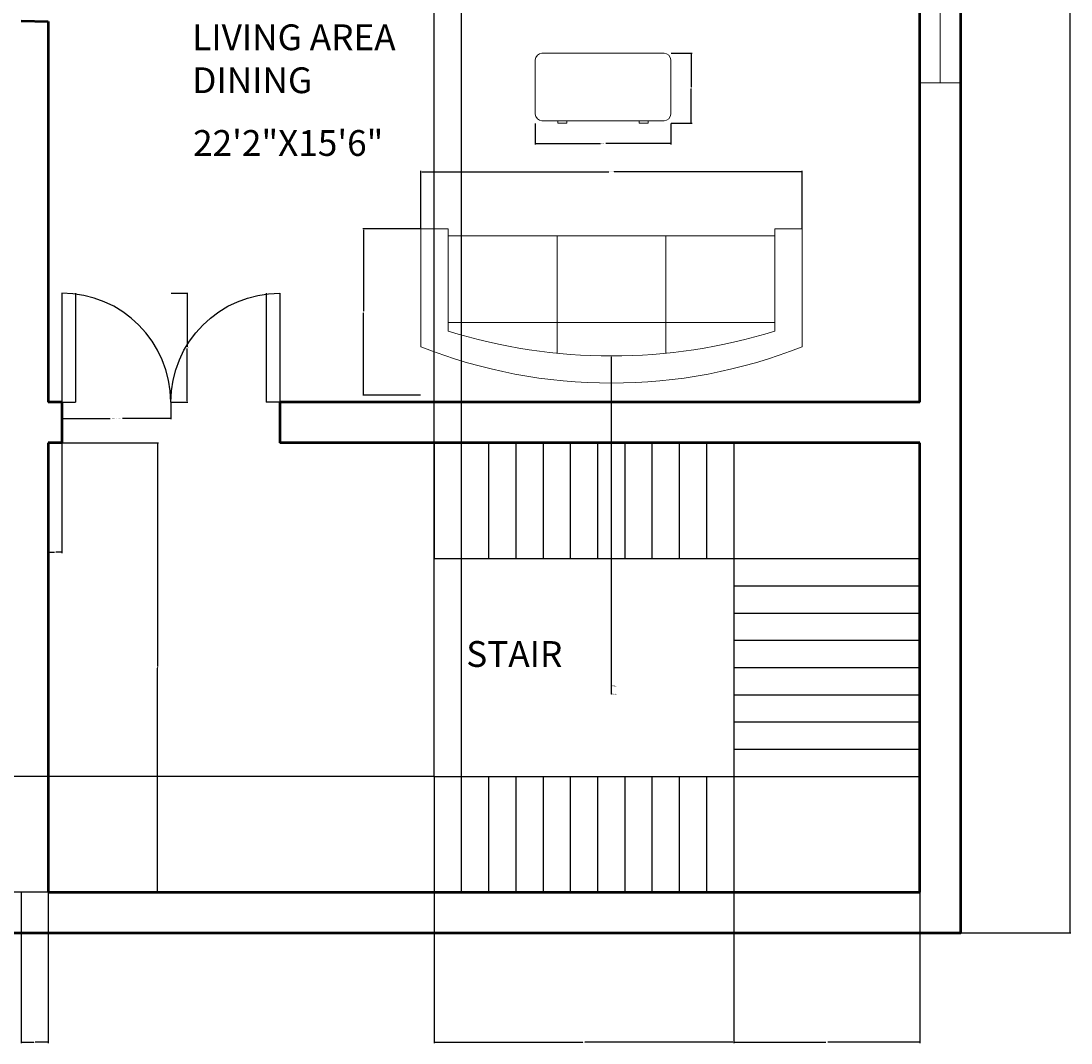
# Model space of a CAD drawing. Units: inches. Extents: x 66 to 499, y 601 to 1111.
# Tile 2 of 4: x 268 to 499, y 601 to 826. Entities that reach past the tile are written whole.
import ezdxf

# ---------------------------------------------------------------- set-up
doc = ezdxf.new("R2010")
doc.units = ezdxf.units.IN
for name, color, linetype, lineweight in [('A-ANNO-DIMS', 2, 'Continuous', 18), ('A-AREA-IDEN', 7, 'Continuous', 18), ('A-DOOR', 3, 'Continuous', 25), ('A-FLOR-STRS', 7, 'Continuous', 25), ('A-FURN', 8, 'Continuous', 18), ('A-GLAZ', 4, 'Continuous', 18), ('A-WALL', 7, 'Continuous', 50)]:
    doc.layers.add(name, color=color, linetype=linetype, lineweight=lineweight)
doc.styles.get("Standard").update_dxf_attribs({"font": 'arial.ttf'})
doc.dimstyles.get("Standard").update_dxf_attribs({"dimtxt": 0.18, "dimasz": 0.18, "dimexe": 0.18, "dimexo": 0.0625, "dimgap": 0.09, "dimtad": 0, "dimtih": 1, "dimtoh": 1, "dimdec": 4, "dimzin": 0, "dimdsep": 46, "dimtxsty": 'Standard', "dimcen": 0.09, "dimadec": 0, "dimazin": 0, "dimtfac": 1, "dimtdec": 4, "dimtofl": 0, "dimtmove": 0, "dimatfit": 3, "dimfxl": 1, "dimtolj": 1, "dimtzin": 0, "dimarcsym": 0})

# ---------------------------------------------------------------- blocks, each defined once
blk = doc.blocks.new('Sofa - Roundback 7 ft.')
for p, q in [((-12.00002, -32.4421), (-12.00003, -6.5971)), ((11.99997, -32.4421), (11.99998, -6.5971)), ((-36.000027, -34), (-36.000027, -11.4696)), ((35.99998, -34), (35.99998, -11.4696)), ((-35.999844, -13.3819), (35.9998, -13.3819)), ((-36.000027, -32.4421), (35.99998, -32.4421))]:
    blk.add_line(p, q)
for points in [[(-36.000027, -34), (-42.000027, -34), (-42.000027, -8)], [(41.99998, -8), (41.99998, -34), (35.99998, -34)]]:
    blk.add_lwpolyline(points)
for centre, radius, start, end in [((0, -114.25), 114.25, 68.43141, 111.5686), ((-0.00001, -127.1968), 121.1968, 72.72033, 107.2797)]:
    blk.add_arc(centre, radius, start, end)
blk = doc.blocks.new('Desk - 30 x 60 in.')
for p, q in [((-26.999995, 0), (26.999995, 0)), ((-29.999995, -27), (-29.999995, -3)), ((29.999995, -3), (29.999995, -27)), ((26.999995, -30), (-26.999995, -30)), ((-20.000005, -30), (-20.000005, -31)), ((-20.000005, -31), (-16.000005, -31)), ((-16.000005, -31), (-16.000005, -30)), ((15.999995, -31), (15.999995, -30)), ((19.999995, -31), (15.999995, -31)), ((19.999995, -30), (19.999995, -31))]:
    blk.add_line(p, q)
for centre, start, end in [((-26.499995, -3.5), 98.1301, 171.8699), ((26.499995, -3.5), 8.130102, 81.8699), ((-26.499995, -26.5), 188.1301, 261.8699), ((26.499995, -26.5), 278.1301, 351.8699)]:
    blk.add_arc(centre, 3.535534, start, end)
blk = doc.blocks.new('DOOR-LEAF-24IN')
for p, q in [((0, 24), (0, 0)), ((3, 24), (3, 0)), ((0, 0), (3, 0))]:
    blk.add_line(p, q)
blk.add_arc((0, 0), 24, 0, 90)
blk = doc.blocks.new('WIN-60IN')
for p, q in [((60, 9), (0, 9)), ((0, 9), (0, 0)), ((60, 0), (60, 9)), ((0, 4.5), (60, 4.5)), ((0, 0), (60, 0))]:
    blk.add_line(p, q)
blk = doc.blocks.new('*D28')
at = {"layer": 'A-ANNO-DIMS', "color": 0, "lineweight": -2, "transparency": 16777216}
for p, q in [((276.58, 741.94), (276.58, 738.22)), ((300.58, 741.94), (300.58, 738.22)), ((276.76, 738.4), (287.24, 738.4)), ((300.4, 738.4), (289.91, 738.4))]:
    blk.add_line(p, q, dxfattribs=at)
at = {"layer": 'A-ANNO-DIMS', "color": 0, "transparency": 16777216}
for points in [[(276.76, 738.43), (276.76, 738.37), (276.58, 738.4)], [(300.4, 738.43), (300.4, 738.37), (300.58, 738.4)]]:
    blk.add_solid(points, dxfattribs=at)
at = {"layer": 'Defpoints', "color": 0, "transparency": 16777216}
for p in [(276.58, 742), (300.58, 742), (300.58, 738.4)]:
    blk.add_point(p, dxfattribs=at)
at = {"layer": 'A-ANNO-DIMS', "color": 0, "transparency": 16777216, "insert": (288.58, 738.4), "char_height": 0.18, "attachment_point": 5}
blk.add_mtext('\\A1;ENTRY LEAF 24 TYP.', dxfattribs=at)
blk = doc.blocks.new('*D29')
at = {"layer": 'A-ANNO-DIMS', "color": 0, "lineweight": -2, "transparency": 16777216}
for p, q in [((300.64, 766), (304.36, 766)), ((304.18, 765.82), (304.18, 754.18)), ((304.18, 742.18), (304.18, 753.82)), ((300.64, 742), (304.36, 742))]:
    blk.add_line(p, q, dxfattribs=at)
at = {"layer": 'A-ANNO-DIMS', "color": 0, "transparency": 16777216}
for points in [[(304.15, 765.82), (304.21, 765.82), (304.18, 766)], [(304.15, 742.18), (304.21, 742.18), (304.18, 742)]]:
    blk.add_solid(points, dxfattribs=at)
at = {"layer": 'Defpoints', "color": 0, "transparency": 16777216}
for p in [(300.58, 766), (304.18, 766), (300.58, 742)]:
    blk.add_point(p, dxfattribs=at)
at = {"layer": 'A-ANNO-DIMS', "color": 0, "transparency": 16777216, "insert": (304.18, 754), "char_height": 0.18, "attachment_point": 5}
blk.add_mtext('\\A1;24 TYP.', dxfattribs=at)
blk = doc.blocks.new('*D34')
at = {"layer": 'A-ANNO-DIMS', "color": 0, "lineweight": -2, "transparency": 16777216}
for p, q in [((355.66, 780.24), (355.66, 792.96)), ((355.84, 792.78), (397.06, 792.78)), ((439.48, 792.78), (398.25, 792.78)), ((439.66, 780.24), (439.66, 792.96))]:
    blk.add_line(p, q, dxfattribs=at)
at = {"layer": 'A-ANNO-DIMS', "color": 0, "transparency": 16777216}
for points in [[(355.84, 792.81), (355.84, 792.75), (355.66, 792.78)], [(439.48, 792.81), (439.48, 792.75), (439.66, 792.78)]]:
    blk.add_solid(points, dxfattribs=at)
at = {"layer": 'Defpoints', "color": 0, "transparency": 16777216}
for p in [(355.66, 792.78), (355.66, 780.18), (439.66, 780.18)]:
    blk.add_point(p, dxfattribs=at)
at = {"layer": 'A-ANNO-DIMS', "color": 0, "transparency": 16777216, "insert": (397.66, 792.78), "char_height": 0.18, "attachment_point": 5}
blk.add_mtext('\\A1;SOFA 84', dxfattribs=at)
blk = doc.blocks.new('*D35')
at = {"layer": 'A-ANNO-DIMS', "color": 0, "lineweight": -2, "transparency": 16777216}
for p, q in [((355.59, 780.18), (342.88, 780.18)), ((343.06, 780), (343.06, 762.03)), ((343.06, 743.7), (343.06, 761.67)), ((355.59, 743.52), (342.88, 743.52))]:
    blk.add_line(p, q, dxfattribs=at)
at = {"layer": 'A-ANNO-DIMS', "color": 0, "transparency": 16777216}
for points in [[(343.03, 780), (343.09, 780), (343.06, 780.18)], [(343.03, 743.7), (343.09, 743.7), (343.06, 743.52)]]:
    blk.add_solid(points, dxfattribs=at)
at = {"layer": 'Defpoints', "color": 0, "transparency": 16777216}
for p in [(355.66, 780.18), (343.06, 743.52), (355.66, 743.52)]:
    blk.add_point(p, dxfattribs=at)
at = {"layer": 'A-ANNO-DIMS', "color": 0, "transparency": 16777216, "insert": (343.06, 761.85), "char_height": 0.18, "attachment_point": 5}
blk.add_mtext('\\A1;37', dxfattribs=at)
blk = doc.blocks.new('*D36')
at = {"layer": 'A-ANNO-DIMS', "color": 0, "lineweight": -2, "transparency": 16777216}
for p, q in [((380.82, 803.4), (380.82, 798.8)), ((410.75, 803.4), (410.75, 798.8)), ((381, 798.98), (395.2, 798.98)), ((410.57, 798.98), (396.38, 798.98))]:
    blk.add_line(p, q, dxfattribs=at)
at = {"layer": 'A-ANNO-DIMS', "color": 0, "transparency": 16777216}
for points in [[(381, 799.01), (381, 798.95), (380.82, 798.98)], [(410.57, 799.01), (410.57, 798.95), (410.75, 798.98)]]:
    blk.add_solid(points, dxfattribs=at)
at = {"layer": 'Defpoints', "color": 0, "transparency": 16777216}
for p in [(380.82, 803.47), (410.75, 803.47), (410.75, 798.98)]:
    blk.add_point(p, dxfattribs=at)
at = {"layer": 'A-ANNO-DIMS', "color": 0, "transparency": 16777216, "insert": (395.79, 798.98), "char_height": 0.18, "attachment_point": 5}
blk.add_mtext('\\A1;DESK 30', dxfattribs=at)
blk = doc.blocks.new('*D37')
at = {"layer": 'A-ANNO-DIMS', "color": 0, "lineweight": -2, "transparency": 16777216}
for p, q in [((410.82, 818.93), (415.42, 818.93)), ((415.24, 818.75), (415.24, 811.38)), ((415.24, 803.65), (415.24, 811.02)), ((410.82, 803.47), (415.42, 803.47))]:
    blk.add_line(p, q, dxfattribs=at)
at = {"layer": 'A-ANNO-DIMS', "color": 0, "transparency": 16777216}
for points in [[(415.21, 818.75), (415.27, 818.75), (415.24, 818.93)], [(415.21, 803.65), (415.27, 803.65), (415.24, 803.47)]]:
    blk.add_solid(points, dxfattribs=at)
at = {"layer": 'Defpoints', "color": 0, "transparency": 16777216}
for p in [(410.75, 818.93), (415.24, 818.93), (410.75, 803.47)]:
    blk.add_point(p, dxfattribs=at)
at = {"layer": 'A-ANNO-DIMS', "color": 0, "transparency": 16777216, "insert": (415.24, 811.2), "char_height": 0.18, "attachment_point": 5}
blk.add_mtext('\\A1;15', dxfattribs=at)
blk = doc.blocks.new('*D43')
at = {"layer": 'A-ANNO-DIMS', "color": 0, "lineweight": -2, "transparency": 16777216}
for p, q in [((474.64, 1087), (498.86, 1087)), ((498.68, 1086.82), (498.68, 856.19)), ((498.68, 625.18), (498.68, 855.82)), ((474.64, 625), (498.86, 625))]:
    blk.add_line(p, q, dxfattribs=at)
at = {"layer": 'A-ANNO-DIMS', "color": 0, "transparency": 16777216}
for points in [[(498.65, 1086.82), (498.71, 1086.82), (498.68, 1087)], [(498.65, 625.18), (498.71, 625.18), (498.68, 625)]]:
    blk.add_solid(points, dxfattribs=at)
at = {"layer": 'Defpoints', "color": 0, "transparency": 16777216}
for p in [(474.58, 1087), (498.68, 1087), (474.58, 625)]:
    blk.add_point(p, dxfattribs=at)
at = {"layer": 'A-ANNO-DIMS', "color": 0, "transparency": 16777216, "insert": (498.68, 856), "char_height": 0.18, "attachment_point": 5}
blk.add_mtext('\\A1;462', dxfattribs=at)
blk = doc.blocks.new('*D51')
at = {"layer": 'A-ANNO-DIMS', "color": 0, "lineweight": -2, "transparency": 16777216}
for p, q in [((273.64, 733), (297.86, 733)), ((297.68, 732.82), (297.68, 683.69)), ((297.68, 634.18), (297.68, 683.32)), ((273.64, 634), (297.86, 634))]:
    blk.add_line(p, q, dxfattribs=at)
at = {"layer": 'A-ANNO-DIMS', "color": 0, "transparency": 16777216}
for points in [[(297.65, 732.82), (297.71, 732.82), (297.68, 733)], [(297.65, 634.18), (297.71, 634.18), (297.68, 634)]]:
    blk.add_solid(points, dxfattribs=at)
at = {"layer": 'Defpoints', "color": 0, "transparency": 16777216}
for p in [(273.58, 733), (273.58, 634), (297.68, 634)]:
    blk.add_point(p, dxfattribs=at)
at = {"layer": 'A-ANNO-DIMS', "color": 0, "transparency": 16777216, "insert": (297.68, 683.5), "char_height": 0.18, "attachment_point": 5}
blk.add_mtext('\\A1;99', dxfattribs=at)
blk = doc.blocks.new('*D52')
at = {"layer": 'A-ANNO-DIMS', "color": 0, "lineweight": -2, "transparency": 16777216}
for p, q in [((358.58, 633.94), (358.58, 600.72)), ((424.58, 633.94), (424.58, 600.72)), ((358.76, 600.9), (391.36, 600.9)), ((424.4, 600.9), (391.8, 600.9))]:
    blk.add_line(p, q, dxfattribs=at)
at = {"layer": 'A-ANNO-DIMS', "color": 0, "transparency": 16777216}
for points in [[(358.76, 600.93), (358.76, 600.87), (358.58, 600.9)], [(424.4, 600.93), (424.4, 600.87), (424.58, 600.9)]]:
    blk.add_solid(points, dxfattribs=at)
at = {"layer": 'Defpoints', "color": 0, "transparency": 16777216}
for p in [(358.58, 634), (424.58, 634), (424.58, 600.9)]:
    blk.add_point(p, dxfattribs=at)
at = {"layer": 'A-ANNO-DIMS', "color": 0, "transparency": 16777216, "insert": (391.58, 600.9), "char_height": 0.18, "attachment_point": 5}
blk.add_mtext('\\A1;66', dxfattribs=at)
blk = doc.blocks.new('*D53')
at = {"layer": 'A-ANNO-DIMS', "color": 0, "lineweight": -2, "transparency": 16777216}
for p, q in [((424.58, 633.94), (424.58, 600.72)), ((465.58, 633.94), (465.58, 600.72)), ((424.76, 600.9), (444.87, 600.9)), ((465.4, 600.9), (445.28, 600.9))]:
    blk.add_line(p, q, dxfattribs=at)
at = {"layer": 'A-ANNO-DIMS', "color": 0, "transparency": 16777216}
for points in [[(424.76, 600.93), (424.76, 600.87), (424.58, 600.9)], [(465.4, 600.93), (465.4, 600.87), (465.58, 600.9)]]:
    blk.add_solid(points, dxfattribs=at)
at = {"layer": 'Defpoints', "color": 0, "transparency": 16777216}
for p in [(424.58, 634), (465.58, 634), (465.58, 600.9)]:
    blk.add_point(p, dxfattribs=at)
at = {"layer": 'A-ANNO-DIMS', "color": 0, "transparency": 16777216, "insert": (445.08, 600.9), "char_height": 0.18, "attachment_point": 5}
blk.add_mtext('\\A1;41', dxfattribs=at)
blk = doc.blocks.new('*D54')
at = {"layer": 'A-ANNO-DIMS', "color": 0, "lineweight": -2, "transparency": 16777216}
for p, q in [((358.51, 659.5), (66.3, 659.5)), ((66.48, 659.32), (66.48, 646.94)), ((66.48, 634.18), (66.48, 646.57)), ((358.51, 634), (66.3, 634))]:
    blk.add_line(p, q, dxfattribs=at)
at = {"layer": 'A-ANNO-DIMS', "color": 0, "transparency": 16777216}
for points in [[(66.45, 659.32), (66.51, 659.32), (66.48, 659.5)], [(66.45, 634.18), (66.51, 634.18), (66.48, 634)]]:
    blk.add_solid(points, dxfattribs=at)
at = {"layer": 'Defpoints', "color": 0, "transparency": 16777216}
for p in [(66.48, 659.5), (358.58, 659.5), (358.58, 634)]:
    blk.add_point(p, dxfattribs=at)
at = {"layer": 'A-ANNO-DIMS', "color": 0, "transparency": 16777216, "insert": (66.48, 646.75), "char_height": 0.18, "attachment_point": 5}
blk.add_mtext('\\A1;25.5', dxfattribs=at)
blk = doc.blocks.new('*D55')
at = {"layer": 'A-ANNO-DIMS', "color": 0, "lineweight": -2, "transparency": 16777216}
for p, q in [((358.58, 659.57), (358.58, 1111.28)), ((358.76, 1111.1), (361.43, 1111.1)), ((364.4, 1111.1), (361.73, 1111.1)), ((364.58, 659.57), (364.58, 1111.28))]:
    blk.add_line(p, q, dxfattribs=at)
at = {"layer": 'A-ANNO-DIMS', "color": 0, "transparency": 16777216}
for points in [[(358.76, 1111.13), (358.76, 1111.07), (358.58, 1111.1)], [(364.4, 1111.13), (364.4, 1111.07), (364.58, 1111.1)]]:
    blk.add_solid(points, dxfattribs=at)
at = {"layer": 'Defpoints', "color": 0, "transparency": 16777216}
for p in [(364.58, 1111.1), (358.58, 659.5), (364.58, 659.5)]:
    blk.add_point(p, dxfattribs=at)
at = {"layer": 'A-ANNO-DIMS', "color": 0, "transparency": 16777216, "insert": (361.58, 1111.1), "char_height": 0.18, "attachment_point": 5}
blk.add_mtext('\\A1;6', dxfattribs=at)
blk = doc.blocks.new('*D62')
at = {"layer": 'A-ANNO-DIMS', "color": 0, "lineweight": -2, "transparency": 16777216}
for p, q in [((267.58, 633.94), (267.58, 600.72)), ((273.58, 633.94), (273.58, 600.72)), ((267.76, 600.9), (270.43, 600.9)), ((273.4, 600.9), (270.73, 600.9))]:
    blk.add_line(p, q, dxfattribs=at)
at = {"layer": 'A-ANNO-DIMS', "color": 0, "transparency": 16777216}
for points in [[(267.76, 600.93), (267.76, 600.87), (267.58, 600.9)], [(273.4, 600.93), (273.4, 600.87), (273.58, 600.9)]]:
    blk.add_solid(points, dxfattribs=at)
at = {"layer": 'Defpoints', "color": 0, "transparency": 16777216}
for p in [(267.58, 634), (273.58, 634), (267.58, 600.9)]:
    blk.add_point(p, dxfattribs=at)
at = {"layer": 'A-ANNO-DIMS', "color": 0, "transparency": 16777216, "insert": (270.58, 600.9), "char_height": 0.18, "attachment_point": 5}
blk.add_mtext('\\A1;6', dxfattribs=at)
blk = doc.blocks.new('*D64')
at = {"layer": 'A-ANNO-DIMS', "color": 0, "lineweight": -2, "transparency": 16777216}
for p, q in [((273.58, 732.94), (273.58, 708.72)), ((276.58, 732.94), (276.58, 708.72)), ((273.76, 708.9), (274.93, 708.9)), ((276.4, 708.9), (275.22, 708.9))]:
    blk.add_line(p, q, dxfattribs=at)
at = {"layer": 'A-ANNO-DIMS', "color": 0, "transparency": 16777216}
for points in [[(273.76, 708.93), (273.76, 708.87), (273.58, 708.9)], [(276.4, 708.93), (276.4, 708.87), (276.58, 708.9)]]:
    blk.add_solid(points, dxfattribs=at)
at = {"layer": 'Defpoints', "color": 0, "transparency": 16777216}
for p in [(273.58, 733), (276.58, 733), (273.58, 708.9)]:
    blk.add_point(p, dxfattribs=at)
at = {"layer": 'A-ANNO-DIMS', "color": 0, "transparency": 16777216, "insert": (275.08, 708.9), "char_height": 0.18, "attachment_point": 5}
blk.add_mtext('\\A1;3', dxfattribs=at)
blk = doc.blocks.new('*D68')
at = {"layer": 'A-ANNO-DIMS', "color": 0, "lineweight": -2, "transparency": 16777216}
for p, q in [((397.57, 873.38), (397.75, 873.38)), ((397.66, 873.29), (397.66, 873.47)), ((397.66, 679.46), (397.66, 752)), ((397.84, 679.46), (397.66, 679.46))]:
    blk.add_line(p, q, dxfattribs=at)
at = {"layer": 'A-ANNO-DIMS', "color": 0, "transparency": 16777216}
blk.add_solid([(397.69, 752), (397.63, 752), (397.66, 752.18)], dxfattribs=at)
at = {"layer": 'Defpoints', "color": 0, "transparency": 16777216}
for p in [(397.66, 873.38), (397.66, 752.18)]:
    blk.add_point(p, dxfattribs=at)
at = {"layer": 'A-ANNO-DIMS', "color": 0, "transparency": 16777216, "insert": (398.32, 679.46), "char_height": 0.18, "attachment_point": 5}
blk.add_mtext('\\A1;R121.2', dxfattribs=at)
blk = doc.blocks.new('*D69')
at = {"layer": 'A-ANNO-DIMS', "color": 0, "lineweight": -2, "transparency": 16777216}
for p, q in [((397.66, 860.34), (397.66, 860.52)), ((397.57, 860.43), (397.75, 860.43)), ((397.66, 677.63), (397.66, 746)), ((397.84, 677.63), (397.66, 677.63))]:
    blk.add_line(p, q, dxfattribs=at)
at = {"layer": 'A-ANNO-DIMS', "color": 0, "transparency": 16777216}
blk.add_solid([(397.69, 746), (397.63, 746), (397.66, 746.18)], dxfattribs=at)
at = {"layer": 'Defpoints', "color": 0, "transparency": 16777216}
for p in [(397.66, 860.43), (397.66, 746.18)]:
    blk.add_point(p, dxfattribs=at)
at = {"layer": 'A-ANNO-DIMS', "color": 0, "transparency": 16777216, "insert": (398.39, 677.63), "char_height": 0.18, "attachment_point": 5}
blk.add_mtext('\\A1;R114.25', dxfattribs=at)

msp = doc.modelspace()

# ---------------------------------------------------------------- linework, layer by layer
at = {"layer": 'A-FLOR-STRS'}
for p, q in [((358.5757, 733.0042), (358.5757, 707.5042)), ((364.5757, 733.0042), (364.5757, 707.5042)), ((370.5757, 733.0042), (370.5757, 707.5042)), ((376.5757, 733.0042), (376.5757, 707.5042)), ((382.5757, 733.0042), (382.5757, 707.5042)), ((388.5757, 733.0042), (388.5757, 707.5042)), ((394.5757, 733.0042), (394.5757, 707.5042)), ((400.5757, 733.0042), (400.5757, 707.5042)), ((406.5757, 733.0042), (406.5757, 707.5042)), ((412.5757, 733.0042), (412.5757, 707.5042)), ((418.5757, 733.0042), (418.5757, 707.5042)), ((424.5757, 733.0042), (424.5757, 634.0042)), ((358.5757, 707.5042), (465.5757, 707.5042)), ((424.5757, 701.5042), (465.5757, 701.5042)), ((424.5757, 695.5042), (465.5757, 695.5042)), ((424.5757, 689.5042), (465.5757, 689.5042)), ((424.5757, 683.5042), (465.5757, 683.5042)), ((424.5757, 677.5042), (465.5757, 677.5042)), ((424.5757, 671.5042), (465.5757, 671.5042)), ((424.5757, 665.5042), (465.5757, 665.5042)), ((358.5757, 659.5042), (465.5757, 659.5042)), ((358.5757, 659.5042), (358.5757, 634.0042)), ((364.5757, 659.5042), (364.5757, 634.0042)), ((370.5757, 659.5042), (370.5757, 634.0042)), ((376.5757, 659.5042), (376.5757, 634.0042)), ((382.5757, 659.5042), (382.5757, 634.0042)), ((388.5757, 659.5042), (388.5757, 634.0042)), ((394.5757, 659.5042), (394.5757, 634.0042)), ((400.5757, 659.5042), (400.5757, 634.0042)), ((406.5757, 659.5042), (406.5757, 634.0042)), ((412.5757, 659.5042), (412.5757, 634.0042)), ((418.5757, 659.5042), (418.5757, 634.0042))]:
    msp.add_line(p, q, dxfattribs=at)
at = {"layer": 'A-WALL'}
for p, q in [((465.5757, 742.0042), (465.5757, 928.0042)), ((267.5757, 826.0042), (273.5757, 825.9236)), ((273.5757, 825.9236), (273.5757, 742.0042)), ((276.5757, 742.0042), (273.5757, 742.0042)), ((276.5757, 742.0042), (276.5757, 733.0042)), ((465.5757, 742.0042), (324.5757, 742.0042)), ((324.5757, 742.0042), (324.5757, 733.0042)), ((276.5757, 733.0042), (273.5757, 733.0042)), ((273.5757, 733.0042), (273.5757, 634.0042)), ((465.5757, 733.0042), (324.5757, 733.0042)), ((465.5757, 634.0042), (465.5757, 733.0042)), ((273.5757, 634.0042), (465.5757, 634.0042))]:
    msp.add_line(p, q, dxfattribs=at)
msp.add_lwpolyline([(90.5757, 625.0042), (474.5757, 625.0042), (474.5757, 1087.0042), (90.5757, 1087.0042)], close=True, dxfattribs=at)

# ---------------------------------------------------------------- block references
at = {"layer": 'A-DOOR'}
msp.add_blockref('DOOR-LEAF-24IN', (276.5757, 742.0042), dxfattribs=at)
at = {"layer": 'A-DOOR', "extrusion": (0, 0, -1), "zscale": -1}
msp.add_blockref('DOOR-LEAF-24IN', (-324.5757, 742.0042), dxfattribs=at)
at = {"layer": 'A-FURN', "xscale": 0.4989042774843635, "yscale": 0.4989042774843635, "zscale": 0.4989042774843635}
msp.add_blockref('Desk - 30 x 60 in.', (395.7875, 818.9331), dxfattribs=at)
at = {"layer": 'A-FURN', "rotation": 180}
msp.add_blockref('Sofa - Roundback 7 ft.', (397.6569, 746.1823), dxfattribs=at)
at = {"layer": 'A-GLAZ', "rotation": 270.0000000000001}
msp.add_blockref('WIN-60IN', (465.5667, 872.3672), dxfattribs=at)

# ---------------------------------------------------------------- texts
at = {"layer": 'A-AREA-IDEN', "attachment_point": 1}
for s, insert, char_height in [('LIVING AREA\\PDINING', (305.2977, 825.2516), 5.682095), ('22\'2"X15\'6"', (305.4798, 801.9492), 5.682095), ('STAIR', (365.6574, 689.3134), 5.6821)]:
    msp.add_mtext_dynamic_manual_height_columns(s, width=58.656418, gutter_width=28.4105, heights=[0], dxfattribs=dict(at, insert=insert, char_height=char_height))

# ---------------------------------------------------------------- dimensions: what is measured, and where the dimension line sits
at = {"layer": 'A-ANNO-DIMS'}
for base, p1, p2, picture, middle in [((364.5757, 1111.1042), (358.5757, 659.5042), (364.5757, 659.5042), '*D55', (361.5757, 1111.1042)), ((267.5757, 600.9042), (273.5757, 634.0042), (267.5757, 634.0042), '*D62', (270.5757, 600.9042)), ((424.5757, 600.9042), (358.5757, 634.0042), (424.5757, 634.0042), '*D52', (391.5757, 600.9042)), ((465.5757, 600.9042), (424.5757, 634.0042), (465.5757, 634.0042), '*D53', (445.0757, 600.9042))]:
    dim = msp.add_linear_dim(base=base, p1=p1, p2=p2, dimstyle='Standard', override={"dimdec": 0, "dimlfac": 1, "dimrnd": 0, "dimzin": 0, "dimdsep": 46, "dimlunit": 2}, dxfattribs=at)
    dim.commit()
    dim.dimension.update_dxf_attribs({"geometry": picture, "text_midpoint": middle})
for base, p1, p2, angle, override, picture, middle in [((498.6757, 1087.0042), (474.5757, 625.0042), (474.5757, 1087.0042), 90, {"dimdec": 0, "dimlfac": 1, "dimrnd": 0, "dimzin": 0, "dimdsep": 46, "dimlunit": 2}, '*D43', (498.6757, 856.0042)), ((415.2447, 818.9331), (410.7546, 803.4671), (410.7546, 818.9331), 90, {"dimdec": 0, "dimlfac": 1, "dimrnd": 0, "dimzin": 0, "dimdsep": 46, "dimlunit": 2}, '*D37', (415.2447, 811.2001)), ((343.0569, 743.5157), (355.6569, 780.1823), (355.6569, 743.5157), 270, {"dimdec": 0, "dimlfac": 1, "dimrnd": 0, "dimzin": 0, "dimdsep": 46, "dimlunit": 2}, '*D35', (343.0569, 761.849)), ((297.6757, 634.0042), (273.5757, 733.0042), (273.5757, 634.0042), 270, {"dimdec": 0, "dimlfac": 1, "dimrnd": 0, "dimzin": 0, "dimdsep": 46, "dimlunit": 2}, '*D51', (297.6757, 683.5042)), ((273.5757, 708.9042), (276.5757, 733.0042), (273.5757, 733.0042), 180, {"dimdec": 0, "dimlfac": 1, "dimrnd": 0, "dimzin": 0, "dimdsep": 46, "dimlunit": 2}, '*D64', (275.0757, 708.9042)), ((66.4757, 659.5042), (358.5757, 634.0042), (358.5757, 659.5042), 90, {"dimdec": 1, "dimlfac": 1, "dimrnd": 0, "dimzin": 0, "dimdsep": 46, "dimlunit": 2}, '*D54', (66.4757, 646.7542))]:
    dim = msp.add_linear_dim(base=base, p1=p1, p2=p2, angle=angle, dimstyle='Standard', override=override, dxfattribs=at)
    dim.commit()
    dim.dimension.update_dxf_attribs({"geometry": picture, "text_midpoint": middle})
for center, mpoint, override, picture, middle in [((397.6569, 873.3791), (397.657, 752.1823), {"dimdec": 1, "dimlfac": 1, "dimrnd": 0, "dimzin": 0, "dimdsep": 46, "dimlunit": 2}, '*D68', (398.316, 679.4643)), ((397.6569, 860.4323), (397.657, 746.1823), {"dimdec": 2, "dimlfac": 1, "dimrnd": 0, "dimzin": 0, "dimdsep": 46, "dimlunit": 2}, '*D69', (398.3875, 677.6323))]:
    dim = msp.add_radius_dim(center=center, mpoint=mpoint, dimstyle='Standard', override=override, dxfattribs=at)
    dim.commit()
    dim.dimension.update_dxf_attribs({"geometry": picture, "text_midpoint": middle, "dimtype": 164})
for base, p1, p2, text, picture, middle in [((410.7546, 798.9769), (380.8204, 803.4671), (410.7546, 803.4671), 'DESK <>', '*D36', (395.7875, 798.9769)), ((300.5757, 738.4042), (276.5757, 742.0042), (300.5757, 742.0042), 'ENTRY LEAF <> TYP.', '*D28', (288.5757, 738.4042))]:
    dim = msp.add_linear_dim(base=base, p1=p1, p2=p2, text=text, dimstyle='Standard', override={"dimdec": 0, "dimlfac": 1, "dimrnd": 0, "dimzin": 0, "dimdsep": 46, "dimlunit": 2}, dxfattribs=at)
    dim.commit()
    dim.dimension.update_dxf_attribs({"geometry": picture, "text_midpoint": middle})
for base, p1, p2, angle, text, picture, middle in [((355.6569, 792.7823), (439.6569, 780.1823), (355.6569, 780.1823), 180, 'SOFA <>', '*D34', (397.6569, 792.7823)), ((304.1757, 766.0042), (300.5757, 742.0042), (300.5757, 766.0042), 90, '<> TYP.', '*D29', (304.1757, 754.0042))]:
    dim = msp.add_linear_dim(base=base, p1=p1, p2=p2, angle=angle, text=text, dimstyle='Standard', override={"dimdec": 0, "dimlfac": 1, "dimrnd": 0, "dimzin": 0, "dimdsep": 46, "dimlunit": 2}, dxfattribs=at)
    dim.commit()
    dim.dimension.update_dxf_attribs({"geometry": picture, "text_midpoint": middle})

doc.saveas('drawing.dxf')
